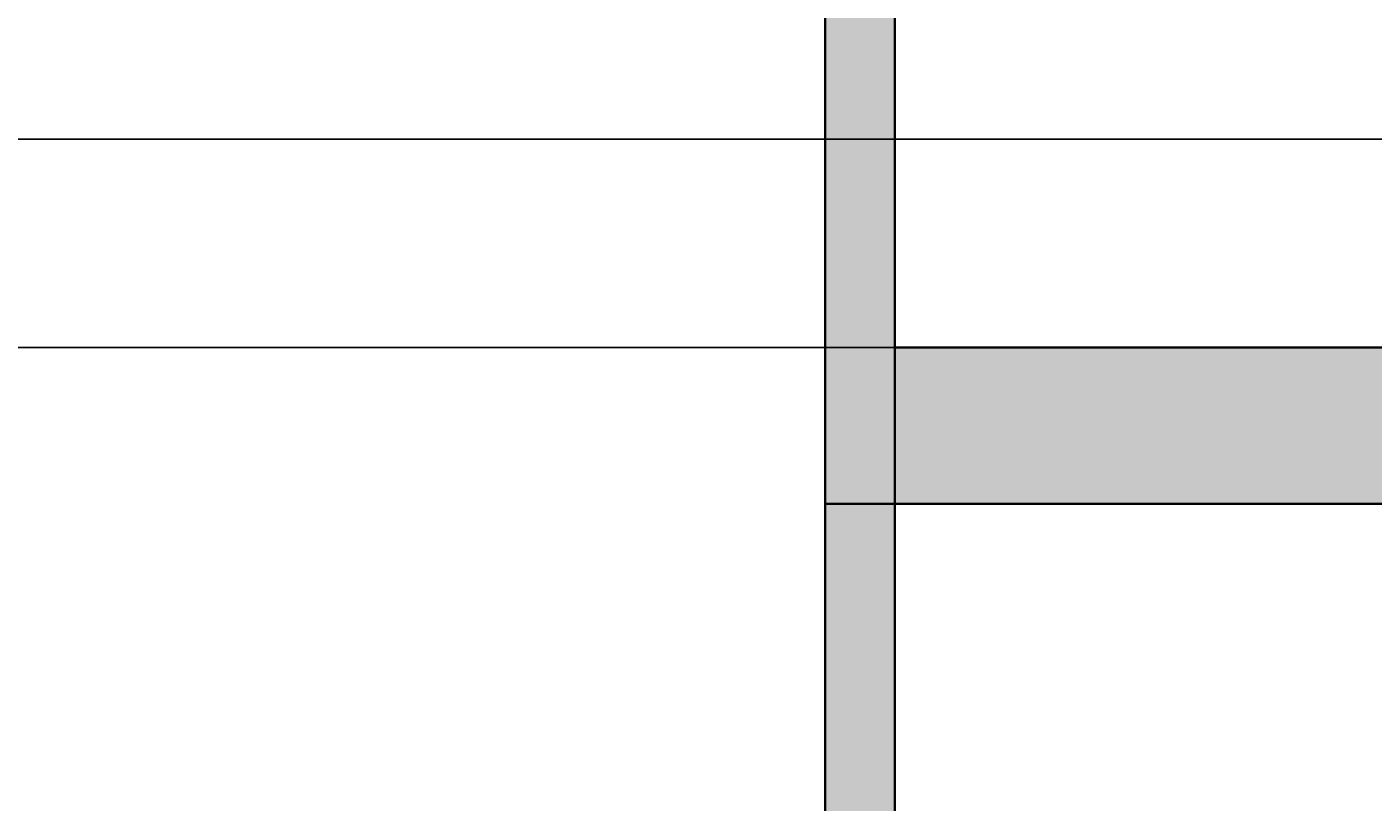
# Model space of a CAD drawing. Units: inches. Extents: x 1998 to 2588, y 1139 to 1977.
# Tile 4 of 134: x 2036 to 2075, y 1576 to 1598. Entities that reach past the tile are written whole.
import ezdxf

# ---------------------------------------------------------------- set-up
doc = ezdxf.new("R2010")
doc.units = ezdxf.units.IN
for name, color, linetype, lineweight in [('A-ANNO-DIMS', 2, 'Continuous', 18), ('A-WALL-PATT', 252, 'Continuous', 13), ('WALL', 200, 'Continuous', 35)]:
    doc.layers.add(name, color=color, linetype=linetype, lineweight=lineweight)
doc.styles.get("Standard").update_dxf_attribs({"font": 'arial.ttf'})
doc.dimstyles.get("Standard").update_dxf_attribs({"dimtxt": 0.18, "dimasz": 0.18, "dimexe": 0.18, "dimexo": 0.0625, "dimgap": 0.09, "dimtad": 0, "dimtih": 1, "dimtoh": 1, "dimdec": 4, "dimzin": 0, "dimdsep": 46, "dimtxsty": 'Standard', "dimcen": 0.09, "dimadec": 0, "dimazin": 0, "dimtfac": 1, "dimtdec": 4, "dimtofl": 0, "dimtmove": 0, "dimatfit": 3, "dimfxl": 1, "dimtolj": 1, "dimtzin": 0, "dimarcsym": 0})

# ---------------------------------------------------------------- blocks, each defined once
blk = doc.blocks.new('*D30')
at = {"layer": 'A-ANNO-DIMS', "color": 0, "lineweight": -2, "transparency": 16777216}
for p, q in [((2407.91, 1636.732), (1997.843, 1636.732)), ((1998.023, 1636.552), (1998.023, 1615.913)), ((1998.023, 1594.912), (1998.023, 1615.552)), ((2407.91, 1594.732), (1997.843, 1594.732))]:
    blk.add_line(p, q, dxfattribs=at)
at = {"layer": 'A-ANNO-DIMS', "color": 0, "transparency": 16777216}
for points in [[(1997.993, 1636.552), (1998.053, 1636.552), (1998.023, 1636.732)], [(1997.993, 1594.912), (1998.053, 1594.912), (1998.023, 1594.732)]]:
    blk.add_solid(points, dxfattribs=at)
at = {"layer": 'Defpoints', "color": 0, "transparency": 16777216}
for p in [(1998.023, 1636.732), (2407.973, 1636.732), (2407.973, 1594.732)]:
    blk.add_point(p, dxfattribs=at)
at = {"layer": 'A-ANNO-DIMS', "color": 0, "transparency": 16777216, "insert": (1998.023, 1615.732), "char_height": 0.18, "attachment_point": 5}
blk.add_mtext('\\A1;42', dxfattribs=at)
blk = doc.blocks.new('*D34')
at = {"layer": 'A-ANNO-DIMS', "color": 0, "lineweight": -2, "transparency": 16777216}
for p, q in [((2407.91, 1594.732), (1997.843, 1594.732)), ((1998.023, 1594.552), (1998.023, 1558.913)), ((1998.023, 1522.912), (1998.023, 1558.552)), ((2407.91, 1522.732), (1997.843, 1522.732))]:
    blk.add_line(p, q, dxfattribs=at)
at = {"layer": 'A-ANNO-DIMS', "color": 0, "transparency": 16777216}
for points in [[(1997.993, 1594.552), (1998.053, 1594.552), (1998.023, 1594.732)], [(1997.993, 1522.912), (1998.053, 1522.912), (1998.023, 1522.732)]]:
    blk.add_solid(points, dxfattribs=at)
at = {"layer": 'Defpoints', "color": 0, "transparency": 16777216}
for p in [(1998.023, 1594.732), (2407.973, 1594.732), (2407.973, 1522.732)]:
    blk.add_point(p, dxfattribs=at)
at = {"layer": 'A-ANNO-DIMS', "color": 0, "transparency": 16777216, "insert": (1998.023, 1558.732), "char_height": 0.18, "attachment_point": 5}
blk.add_mtext('\\A1;72', dxfattribs=at)
blk = doc.blocks.new('*D35')
at = {"layer": 'A-ANNO-DIMS', "color": 0, "lineweight": -2, "transparency": 16777216}
for p, q in [((2148.392, 1612.732), (1997.843, 1612.732)), ((1998.023, 1612.552), (1998.023, 1600.913)), ((1998.023, 1588.912), (1998.023, 1600.552)), ((2148.392, 1588.732), (1997.843, 1588.732))]:
    blk.add_line(p, q, dxfattribs=at)
at = {"layer": 'A-ANNO-DIMS', "color": 0, "transparency": 16777216}
for points in [[(1997.993, 1612.552), (1998.053, 1612.552), (1998.023, 1612.732)], [(1997.993, 1588.912), (1998.053, 1588.912), (1998.023, 1588.732)]]:
    blk.add_solid(points, dxfattribs=at)
at = {"layer": 'Defpoints', "color": 0, "transparency": 16777216}
for p in [(1998.023, 1612.732), (2148.455, 1612.732), (2148.455, 1588.732)]:
    blk.add_point(p, dxfattribs=at)
at = {"layer": 'A-ANNO-DIMS', "color": 0, "transparency": 16777216, "insert": (1998.023, 1600.732), "char_height": 0.18, "attachment_point": 5}
blk.add_mtext('\\A1;24', dxfattribs=at)

msp = doc.modelspace()

# ---------------------------------------------------------------- hatches: boundary and pattern name
at = {"layer": 'A-WALL-PATT'}
h = msp.add_hatch(color=256, dxfattribs=at)
h.dxf.hatch_style = 1
h.paths.add_polyline_path([(2227.4729, 1911.2324), (2222.9729, 1911.2324), (2222.9729, 1888.7324), (2227.4729, 1888.7324)])
h.paths.add_polyline_path([(2236.4493, 1870.3636), (2236.4493, 1875.2324), (2234.4125, 1875.2324), (2234.4125, 1868.3278), (2227.4729, 1868.3278), (2227.4729, 1866.2324), (2236.4493, 1866.2324)])
h.paths.add_polyline_path([(2330.0332, 1875.2324), (2263.9907, 1875.2324), (2263.9907, 1866.2324), (2330.0332, 1866.2324)])
h.paths.add_polyline_path([(2345.9729, 1906.7324), (2393.9729, 1906.7324), (2393.9729, 1882.7324), (2345.9729, 1882.7324), (2345.9729, 1878.2324), (2393.9729, 1878.2324), (2398.4729, 1878.2324), (2398.4729, 1882.7324), (2398.4729, 1911.2324), (2345.9729, 1911.2324), (2341.4729, 1911.2324), (2341.4729, 1866.2324), (2341.4729, 1790.0412), (2345.9729, 1790.0412), (2345.9729, 1875.2324)])
h.paths.add_polyline_path([(2398.4729, 1878.2324), (2393.9729, 1878.2324), (2393.9729, 1798.2324), (2393.9729, 1793.7324), (2398.4729, 1793.7324)], flags=17)
h.paths.add_polyline_path([(2393.9729, 1798.2324), (2375.7311, 1798.2324, -0.005968), (2375.7384, 1797.6146), (2375.7384, 1793.7324), (2393.9729, 1793.7324)], flags=17)
h.paths.add_polyline_path([(2349.8569, 1797.6146), (2349.8569, 1798.2324), (2345.9729, 1798.2324), (2345.9729, 1793.7324), (2349.8569, 1793.7324)], flags=17)
h.paths.add_polyline_path([(2398.4729, 1793.7324), (2393.9729, 1793.7324), (2393.9729, 1790.0412), (2398.4729, 1790.0412)], flags=17)
h.paths.add_polyline_path([(2527.4729, 1882.7324), (2507.8006, 1882.7324), (2507.8006, 1878.2324), (2518.4729, 1878.2324), (2518.4729, 1759.7324), (2510.9729, 1759.7324), (2510.9729, 1755.2324), (2527.4729, 1755.2324)])
h.paths.add_polyline_path([(2487.396, 1882.7324), (2398.4729, 1882.7324), (2398.4729, 1878.2324), (2487.396, 1878.2324)])
h.paths.add_polyline_path([(2490.5682, 1759.7324), (2345.9729, 1759.7324), (2345.9729, 1755.2324), (2490.5682, 1755.2324)])
h.paths.add_polyline_path([(2398.4729, 1760.5844), (2398.3914, 1760.5844), (2393.9729, 1760.5844), (2393.9729, 1759.7324), (2398.4729, 1759.7324)])
h.paths.add_polyline_path([(2334.5332, 1759.7324), (2234.4125, 1759.7324), (2234.4125, 1755.2324), (2334.5332, 1755.2324)])
h.paths.add_polyline_path([(2345.9729, 1760.5844), (2341.5543, 1760.5844), (2341.4729, 1760.5844), (2341.4729, 1759.7324), (2345.9729, 1759.7324)])
h.paths.add_polyline_path([(2222.9729, 1759.7324), (2221.7204, 1759.7324), (2221.7204, 1755.2324), (2222.9729, 1755.2324)])
h.paths.add_polyline_path([(2061.4729, 1702.7324), (2059.4729, 1702.7324), (2059.4729, 1584.2324), (2061.4729, 1584.2324)])
h.paths.add_polyline_path([(2061.4729, 1584.2324), (2059.4729, 1584.2324), (2059.4729, 1470.2324), (2061.4729, 1470.2324)])
h.paths.add_polyline_path([(2510.9729, 1469.2927), (2501.9729, 1469.2927), (2501.9729, 1369.172), (2510.9729, 1369.172)])
h.paths.add_polyline_path([(2227.4729, 1369.7324), (2227.4729, 1417.7324), (2221.4126, 1417.7324), (2221.4126, 1413.2324), (2222.9729, 1413.2324), (2222.9729, 1293.2324), (2222.9729, 1285.137), (2227.4729, 1285.137)])
h = msp.add_hatch(color=256, dxfattribs=at)
h.dxf.hatch_style = 1
h.paths.add_polyline_path([(2222.9729, 1888.7324), (2099.4125, 1888.7324), (2099.4125, 1879.7324), (2222.9729, 1879.7324)])
h.paths.add_polyline_path([(2096.9729, 1868.3278), (2087.9729, 1868.3278), (2087.9729, 1775.637), (2096.9729, 1775.637)])
h.paths.add_polyline_path([(2227.4729, 1868.3278), (2222.9729, 1868.3278), (2222.9729, 1774.3318), (2227.4729, 1774.3318)])
h.paths.add_polyline_path([(2188.3019, 1759.7324), (2138.6074, 1759.7324), (2099.4125, 1759.7324), (2099.4125, 1755.2324), (2176.9729, 1755.2324), (2188.3019, 1755.2324)])
h.paths.add_polyline_path([(2087.9729, 1759.7324), (2059.4729, 1759.7324), (2059.4729, 1702.7324), (2087.9729, 1702.7324), (2087.9729, 1707.2324), (2063.9729, 1707.2324), (2063.9729, 1755.2324), (2087.9729, 1755.2324)])
h.paths.add_polyline_path([(2096.9729, 1755.2324), (2087.9729, 1755.2324), (2087.9729, 1707.2324), (2096.9729, 1707.2324)])
h.paths.add_polyline_path([(2187.0461, 1707.2324), (2105.9729, 1707.2324), (2096.9729, 1707.2324), (2087.9729, 1707.2324), (2087.9729, 1702.7324), (2105.9729, 1702.7324), (2114.9729, 1702.7324), (2187.0461, 1702.7324)])
h.paths.add_polyline_path([(2181.4729, 1719.2028), (2176.9729, 1719.2028), (2176.9729, 1707.2324), (2181.4729, 1707.2324)])
h.paths.add_polyline_path([(2216.0332, 1588.7324), (2114.9729, 1588.7324), (2105.9729, 1588.7324), (2105.9729, 1584.2324), (2216.0332, 1584.2324)])
h.paths.add_polyline_path([(2077.691, 1588.7324), (2061.4729, 1588.7324), (2061.4729, 1584.2324), (2077.691, 1584.2324)])
h.paths.add_polyline_path([(2105.9729, 1588.7324), (2098.0956, 1588.7324), (2098.0956, 1584.2324), (2105.9729, 1584.2324)])
h.paths.add_polyline_path([(2114.9729, 1596.2642), (2110.1012, 1596.2642), (2105.9729, 1596.2642), (2105.9729, 1588.7324), (2114.9729, 1588.7324)])
h.paths.add_polyline_path([(2114.9729, 1584.2324), (2105.9729, 1584.2324), (2105.9729, 1580.249), (2110.1012, 1580.249), (2114.9729, 1580.249)])
h.paths.add_polyline_path([(2114.9729, 1547.7716), (2110.1012, 1547.7716, -0.0318759), (2105.9729, 1548.035), (2105.9729, 1470.2324), (2108.3775, 1470.2324), (2108.3775, 1465.7324), (2186.2943, 1465.7324), (2186.2943, 1470.2324), (2114.9729, 1470.2324)])
h.paths.add_polyline_path([(2227.4729, 1584.2324), (2222.9729, 1584.2324), (2222.9729, 1486.137), (2227.4729, 1486.137)])
h.paths.add_polyline_path([(2295.4138, 1593.2324), (2227.4729, 1593.2324), (2227.4729, 1588.7324), (2295.4138, 1588.7324), (2295.4138, 1591.8729)])
h.paths.add_polyline_path([(2345.9729, 1627.1165), (2341.4729, 1627.1165), (2341.4729, 1593.2324), (2337.2869, 1593.2324), (2337.2869, 1591.8729), (2337.2869, 1588.7324), (2345.9729, 1588.7324)])
h.paths.add_polyline_path([(2291.9729, 1588.7324), (2287.4729, 1588.7324), (2287.4729, 1522.7324), (2291.9729, 1522.7324)])
h.paths.add_polyline_path([(2291.9729, 1522.7324), (2287.4729, 1522.7324), (2227.4729, 1522.7324), (2227.4729, 1518.2324), (2291.9729, 1518.2324)])
h.paths.add_polyline_path([(2295.7347, 1519.5919), (2295.7347, 1522.7324), (2291.9729, 1522.7324), (2291.9729, 1518.2324), (2295.7347, 1518.2324)])
h.paths.add_polyline_path([(2345.9729, 1522.7324), (2337.6078, 1522.7324), (2337.6078, 1519.5919), (2337.6078, 1518.2324), (2341.4729, 1518.2324), (2341.4729, 1488.5616), (2345.9729, 1488.5616)])
h.paths.add_polyline_path([(2345.9729, 1468.1569), (2341.4729, 1468.1569), (2341.4729, 1374.2324), (2227.4729, 1374.2324), (2227.4729, 1369.7324), (2345.9729, 1369.7324)])
h.paths.add_polyline_path([(2345.9729, 1369.7324), (2341.4729, 1369.7324), (2341.4729, 1362.2324), (2345.9729, 1362.2324)])
h.paths.add_polyline_path([(2345.9729, 1317.7324), (2345.9729, 1322.2324), (2341.4729, 1322.2324), (2341.4729, 1285.137), (2345.9729, 1285.137)], flags=17)
h.paths.add_polyline_path([(2356.2096, 1322.2324), (2345.9729, 1322.2324), (2345.9729, 1317.7324), (2356.2096, 1317.7324), (2356.2096, 1319.3088)], flags=17)
h.paths.add_polyline_path([(2393.9729, 1322.2324), (2375.6999, 1322.2324), (2375.6999, 1319.3088, -0.0202458), (2375.636, 1317.7324), (2393.9729, 1317.7324)], flags=17)
h.paths.add_polyline_path([(2398.4729, 1322.2324), (2393.9729, 1322.2324), (2393.9729, 1317.7324), (2393.9729, 1237.7324), (2345.9729, 1237.7324), (2345.9729, 1264.7324), (2341.4729, 1264.7324), (2341.4729, 1228.7324), (2393.9729, 1228.7324), (2482.7412, 1228.7324), (2482.7412, 1237.7324), (2398.4729, 1237.7324), (2398.4729, 1297.1029)])
h.paths.add_polyline_path([(2398.4729, 1362.2324), (2393.9729, 1362.2324), (2393.9729, 1357.7324), (2398.4729, 1357.7324)])
h.paths.add_polyline_path([(2345.9729, 1329.7549), (2341.4729, 1329.7549), (2341.4729, 1322.2324), (2345.9729, 1322.2324)])

# ---------------------------------------------------------------- linework, layer by layer
at = {"layer": 'WALL'}
for p, q in [((2061.4729, 1473.2749), (2061.4729, 1705.7749)), ((2059.4729, 1470.2324), (2059.4729, 1702.7324)), ((2077.691, 1588.7324), (2061.4729, 1588.7324)), ((2077.691, 1584.2324), (2061.4729, 1584.2324))]:
    msp.add_line(p, q, dxfattribs=at)
for points in [[(2059.4729, 1584.2324), (2061.4729, 1584.2324), (2061.4729, 1702.7324), (2059.4729, 1702.7324)], [(2059.4729, 1470.2324), (2061.4729, 1470.2324), (2061.4729, 1584.2324), (2059.4729, 1584.2324)]]:
    msp.add_lwpolyline(points, close=True, dxfattribs=at)

# ---------------------------------------------------------------- dimensions: what is measured, and where the dimension line sits
at = {"layer": 'A-ANNO-DIMS'}
for base, p1, p2, picture, middle in [((1998.0229, 1636.7324), (2407.9729, 1594.7324), (2407.9729, 1636.7324), '*D30', (1998.0229, 1615.7324)), ((1998.0229, 1612.7324), (2148.4548, 1588.7324), (2148.4548, 1612.7324), '*D35', (1998.0229, 1600.7324)), ((1998.0229, 1594.7324), (2407.9729, 1522.7324), (2407.9729, 1594.7324), '*D34', (1998.0229, 1558.7324))]:
    dim = msp.add_linear_dim(base=base, p1=p1, p2=p2, angle=90, dimstyle='Standard', override={"dimdec": 0, "dimlfac": 1, "dimrnd": 0, "dimzin": 0, "dimdsep": 46, "dimlunit": 2}, dxfattribs=at)
    dim.commit()
    dim.dimension.update_dxf_attribs({"geometry": picture, "text_midpoint": middle})

doc.saveas('drawing.dxf')
